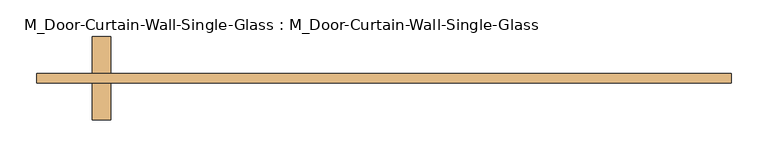
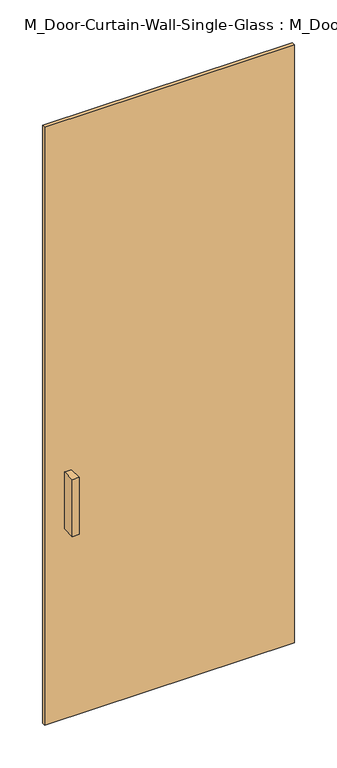
"""IFC4 building model written with IfcOpenShell, lengths in millimetres: door geometry, M_Door-Curtain-Wall-Single-Glass : M_Door-Curtain-Wall-Single-Glass."""

from ifc_helpers import new_model, si_unit, frame, origin, origin_with_axes, place, context, project, spatial, polyline, outline, extrude, source, transform, mapped, element, save


def m_door_curtain_wall_single_glass_m_door_curtain_wall_single_b00c2793(model_context):
    return source(origin(), model_context, "Body", "SweptSolid", [
        extrude(outline(polyline([(475.0, -50.8), (-475.0, -50.8), (-475.0, -38.1), (475.0, -38.1), (475.0, -50.8)])), origin_with_axes(), (0.0, 0.0, 1.0), 2400.0),
        extrude(outline(polyline([(-398.8, -101.6), (-398.8, -50.8), (-373.4, -50.8), (-373.4, -101.6), (-398.8, -101.6)])), frame((0.0, 0.0, 762.0), z_axis=(0.0, 0.0, 1.0), x_axis=(1.0, 0.0, 0.0)), (0.0, 0.0, 1.0), 228.6),
        extrude(outline(polyline([(-373.4, 12.7), (-373.4, -38.1), (-398.8, -38.1), (-398.8, 12.7), (-373.4, 12.7)])), frame((0.0, 0.0, 762.0), z_axis=(0.0, 0.0, 1.0), x_axis=(1.0, 0.0, 0.0)), (0.0, 0.0, 1.0), 228.6),
    ])


if __name__ == "__main__":
    model = new_model("IFC4")
    model_context = context("Model", 3, world=origin())
    ifc_project = project(units=[si_unit("LENGTHUNIT", "METRE", prefix="MILLI")], contexts=[model_context])
    site = spatial("IfcSite", under=ifc_project)
    building = spatial("IfcBuilding", under=site)
    placement = place(None, origin())
    m_door_curtain_wall_single_glass_m_door_curtain_wall_single_shape = m_door_curtain_wall_single_glass_m_door_curtain_wall_single_b00c2793(model_context)
    element("IfcDoor", 1, ObjectType="M_Door-Curtain-Wall-Single-Glass : M_Door-Curtain-Wall-Single-Glass", at=placement, inside=building, context=model_context, shape_type="MappedRepresentation", body=[
        mapped(m_door_curtain_wall_single_glass_m_door_curtain_wall_single_shape, transform((0.0, 0.0, 0.0), x_axis=(1.0, 0.0, 0.0), y_axis=(0.0, 1.0, 0.0), z_axis=(0.0, 0.0, 1.0))),
    ])
    save(model, "model.ifc")

# Revit data of these elements
# Type "M_Door-Curtain-Wall-Single-Glass : M_Door-Curtain-Wall-Single-Glass"
#   Type Mark = "46"
#   Assembly Code = "B2030100"
#   Analytic Construction = "<None>"
#   Width [instance default] = 900 mm
#   Thermal Resistance (R) = 1.7611 (m²·K)/W
#   Swing Angle [instance default] = 90.00°
#   Heat Transfer Coefficient (U) = 0.567826 W/(m²·K)
#   Offset = 50.8 mm
#   Define Thermal Properties by = 1
#   Function = 1
#   Door Handle Material = Aluminum
#   Glazing = Glass
#   Visual Light Transmittance = 0
#   Solar Heat Gain Coefficient = 0
#   Construction Type Id = ""
# Element 1 (IfcDoor, "M_Door-Curtain-Wall-Single-Glass : M_Door-Curtain-Wall-Single-Glass")
#   Width = 950 mm
#   Materials on its faces: "Aluminum", "Glass"
# Materials
#   "Aluminum": class "Metal", colour RGB 247 247 247, transparency 0, Description = "Aluminum 6061", Cost = 0
#   "Glass": class "Glass", colour RGB 0 128 192, transparency 0.9, Description = "Soda Lime Glass", Cost = 0
